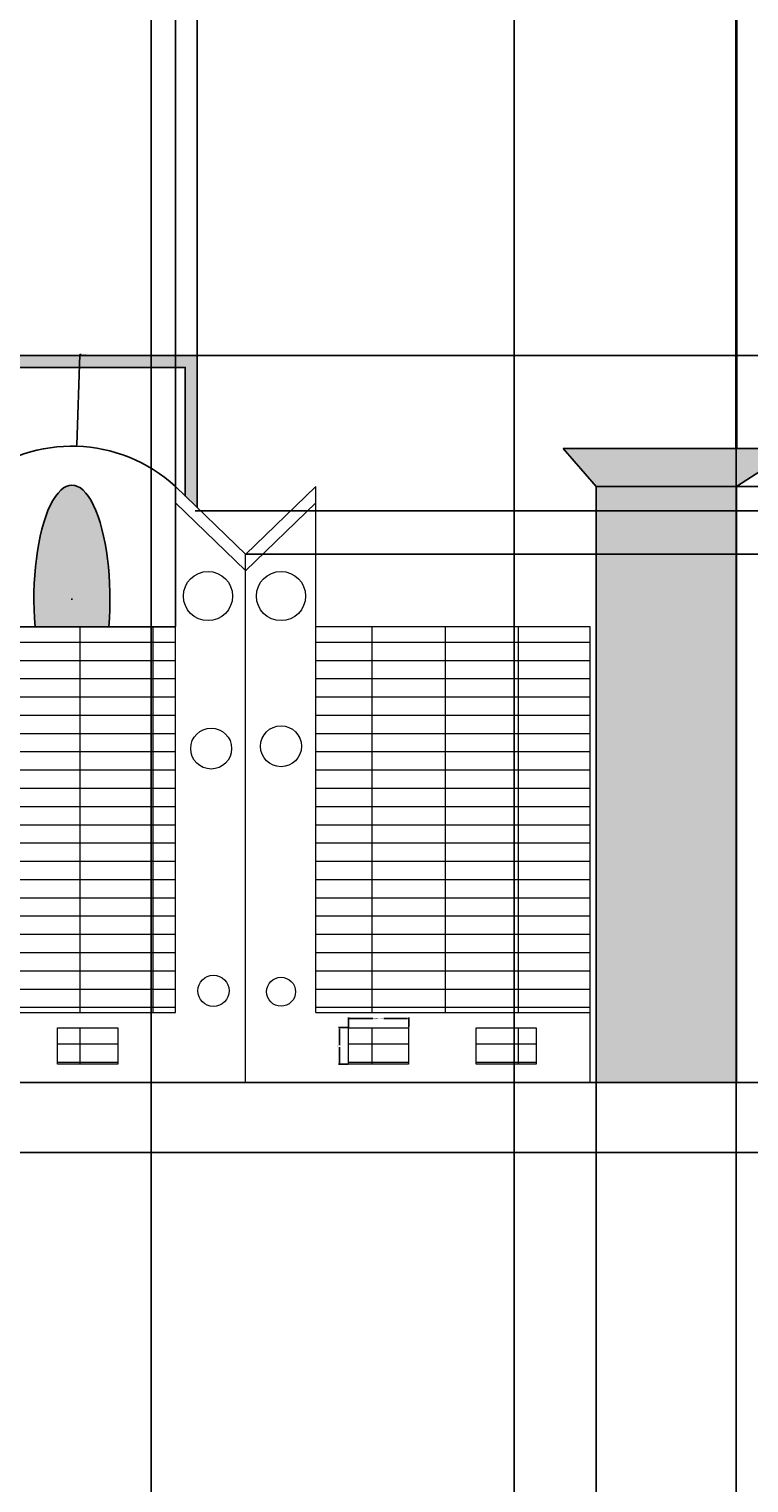
# Model space of a CAD drawing. Units: inches. Extents: x 484 to 1264, y 95 to 991.
# Tile 5 of 8: x 879 to 1002, y 250 to 499. Entities that reach past the tile are written whole.
import ezdxf

# ---------------------------------------------------------------- set-up
doc = ezdxf.new("R2010")
doc.units = ezdxf.units.IN
doc.header["$MEASUREMENT"] = 0
for name, color, linetype, lineweight in [('A-ANNO-DIMS', 2, 'Continuous', 18), ('A-DOOR', 7, 'Continuous', 25), ('A-WALL', 7, 'Continuous', 35), ('L-FENC', 7, 'Continuous', 25), ('L-FENC-GRIL-PATT', 6, 'Continuous', 13), ('L-GATE', 7, 'Continuous', 18)]:
    doc.layers.add(name, color=color, linetype=linetype, lineweight=lineweight)
doc.layers.add('A-ELEV-TRIM-PATT', color=40, linetype='Continuous', lineweight=13, true_color=0xe7c208)
doc.layers.add('L-FENC-PATT', color=34, linetype='Continuous', lineweight=13, true_color=0xa25420)
doc.styles.get("Standard").update_dxf_attribs({"font": 'arial.ttf'})
doc.dimstyles.get("Standard").update_dxf_attribs({"dimtxt": 0.18, "dimasz": 0.18, "dimexe": 0.18, "dimexo": 0.0625, "dimgap": 0.09, "dimtad": 0, "dimtih": 1, "dimtoh": 1, "dimdec": 4, "dimzin": 0, "dimdsep": 46, "dimtxsty": 'Standard', "dimcen": 0.09, "dimadec": 0, "dimazin": 0, "dimtfac": 1, "dimtdec": 4, "dimtofl": 0, "dimtmove": 0, "dimatfit": 3, "dimfxl": 1, "dimtolj": 1, "dimtzin": 0, "dimarcsym": 0})

# ---------------------------------------------------------------- blocks, each defined once
blk = doc.blocks.new('FENCE-PIER-CAP')
for p, q in [((5.63, 0), (0, 6.48)), ((0, 6.48), (39.71, 6.48)), ((39.71, 6.48), (29.63, 0))]:
    blk.add_line(p, q)
blk = doc.blocks.new('GATE-LOWER-INSET')
blk.add_lwpolyline([(0, 6.26), (10.31, 6.26), (10.31, 0), (0, 0)], close=True)
blk = doc.blocks.new('*D8')
at = {"layer": 'A-ANNO-DIMS', "color": 0, "lineweight": -2, "transparency": 16777216}
for p, q in [((933.42, 327.83), (933.42, 329.49)), ((933.6, 329.31), (937.65, 329.31)), ((943.55, 329.31), (939.5, 329.31)), ((943.73, 327.83), (943.73, 329.49))]:
    blk.add_line(p, q, dxfattribs=at)
at = {"layer": 'A-ANNO-DIMS', "color": 0, "transparency": 16777216}
for points in [[(933.6, 329.34), (933.6, 329.28), (933.42, 329.31)], [(943.55, 329.34), (943.55, 329.28), (943.73, 329.31)]]:
    blk.add_solid(points, dxfattribs=at)
at = {"layer": 'Defpoints', "color": 0, "transparency": 16777216}
for p in [(943.73, 329.31), (933.42, 327.77), (943.73, 327.77)]:
    blk.add_point(p, dxfattribs=at)
at = {"layer": 'A-ANNO-DIMS', "color": 0, "transparency": 16777216, "insert": (938.57, 329.31), "char_height": 0.18, "attachment_point": 5}
blk.add_mtext('\\A1;INSET 10 TYP.', dxfattribs=at)
blk = doc.blocks.new('*D9')
at = {"layer": 'A-ANNO-DIMS', "color": 0, "lineweight": -2, "transparency": 16777216}
for p, q in [((933.35, 327.77), (931.69, 327.77)), ((931.87, 327.59), (931.87, 324.82)), ((931.87, 321.68), (931.87, 324.45)), ((933.35, 321.5), (931.69, 321.5))]:
    blk.add_line(p, q, dxfattribs=at)
at = {"layer": 'A-ANNO-DIMS', "color": 0, "transparency": 16777216}
for points in [[(931.84, 327.59), (931.9, 327.59), (931.87, 327.77)], [(931.84, 321.68), (931.9, 321.68), (931.87, 321.5)]]:
    blk.add_solid(points, dxfattribs=at)
at = {"layer": 'Defpoints', "color": 0, "transparency": 16777216}
for p in [(931.87, 327.77), (933.42, 327.77), (933.42, 321.5)]:
    blk.add_point(p, dxfattribs=at)
at = {"layer": 'A-ANNO-DIMS', "color": 0, "transparency": 16777216, "insert": (931.87, 324.63), "char_height": 0.18, "attachment_point": 5}
blk.add_mtext('\\A1;6 TYP.', dxfattribs=at)
blk = doc.blocks.new('*D16')
at = {"layer": 'A-ANNO-DIMS', "color": 0, "lineweight": -2, "transparency": 16777216}
for p, q in [((639.81, 408.32), (639.81, 94.79)), ((999.81, 318.32), (999.81, 94.79)), ((639.99, 94.97), (819.53, 94.97)), ((999.63, 94.97), (820.1, 94.97))]:
    blk.add_line(p, q, dxfattribs=at)
at = {"layer": 'A-ANNO-DIMS', "color": 0, "transparency": 16777216}
for points in [[(639.99, 95), (639.99, 94.94), (639.81, 94.97)], [(999.63, 95), (999.63, 94.94), (999.81, 94.97)]]:
    blk.add_solid(points, dxfattribs=at)
at = {"layer": 'Defpoints', "color": 0, "transparency": 16777216}
for p in [(639.81, 408.38), (999.81, 318.38), (999.81, 94.97)]:
    blk.add_point(p, dxfattribs=at)
at = {"layer": 'A-ANNO-DIMS', "color": 0, "transparency": 16777216, "insert": (819.81, 94.97), "char_height": 0.18, "attachment_point": 5}
blk.add_mtext('\\A1;360', dxfattribs=at)
blk = doc.blocks.new('*D18')
at = {"layer": 'A-ANNO-DIMS', "color": 0, "lineweight": -2, "transparency": 16777216}
for p, q in [((999.88, 501.38), (1264.08, 501.38)), ((1263.9, 501.2), (1263.9, 404.07)), ((1263.9, 306.56), (1263.9, 403.7)), ((595.38, 306.38), (1264.08, 306.38))]:
    blk.add_line(p, q, dxfattribs=at)
at = {"layer": 'A-ANNO-DIMS', "color": 0, "transparency": 16777216}
for points in [[(1263.87, 501.2), (1263.93, 501.2), (1263.9, 501.38)], [(1263.87, 306.56), (1263.93, 306.56), (1263.9, 306.38)]]:
    blk.add_solid(points, dxfattribs=at)
at = {"layer": 'Defpoints', "color": 0, "transparency": 16777216}
for p in [(999.81, 501.38), (1263.9, 501.38), (595.32, 306.38)]:
    blk.add_point(p, dxfattribs=at)
at = {"layer": 'A-ANNO-DIMS', "color": 0, "transparency": 16777216, "insert": (1263.9, 403.88), "char_height": 0.18, "attachment_point": 5}
blk.add_mtext('\\A1;195', dxfattribs=at)
blk = doc.blocks.new('*D40')
at = {"layer": 'A-ANNO-DIMS', "color": 0, "lineweight": -2, "transparency": 16777216}
for p, q in [((899.68, 562.19), (899.68, 94.79)), ((961.76, 562.19), (961.76, 94.79)), ((899.86, 94.97), (930.33, 94.97)), ((961.58, 94.97), (931.12, 94.97))]:
    blk.add_line(p, q, dxfattribs=at)
at = {"layer": 'A-ANNO-DIMS', "color": 0, "transparency": 16777216}
for points in [[(899.86, 95), (899.86, 94.94), (899.68, 94.97)], [(961.58, 95), (961.58, 94.94), (961.76, 94.97)]]:
    blk.add_solid(points, dxfattribs=at)
at = {"layer": 'Defpoints', "color": 0, "transparency": 16777216}
for p in [(899.68, 562.26), (961.76, 562.26), (961.76, 94.97)]:
    blk.add_point(p, dxfattribs=at)
at = {"layer": 'A-ANNO-DIMS', "color": 0, "transparency": 16777216, "insert": (930.72, 94.97), "char_height": 0.18, "attachment_point": 5}
blk.add_mtext('\\A1;62.08', dxfattribs=at)
blk = doc.blocks.new('*D41')
at = {"layer": 'A-ANNO-DIMS', "color": 0, "lineweight": -2, "transparency": 16777216}
for p, q in [((961.76, 562.19), (961.76, 94.79)), ((999.81, 537.32), (999.81, 94.79)), ((961.94, 94.97), (980.39, 94.97)), ((999.63, 94.97), (981.18, 94.97))]:
    blk.add_line(p, q, dxfattribs=at)
at = {"layer": 'A-ANNO-DIMS', "color": 0, "transparency": 16777216}
for points in [[(961.94, 95), (961.94, 94.94), (961.76, 94.97)], [(999.63, 95), (999.63, 94.94), (999.81, 94.97)]]:
    blk.add_solid(points, dxfattribs=at)
at = {"layer": 'Defpoints', "color": 0, "transparency": 16777216}
for p in [(961.76, 562.26), (999.81, 537.38), (999.81, 94.97)]:
    blk.add_point(p, dxfattribs=at)
at = {"layer": 'A-ANNO-DIMS', "color": 0, "transparency": 16777216, "insert": (980.79, 94.97), "char_height": 0.18, "attachment_point": 5}
blk.add_mtext('\\A1;38.05', dxfattribs=at)
blk = doc.blocks.new('*D49')
at = {"layer": 'A-ANNO-DIMS', "color": 0, "lineweight": -2, "transparency": 16777216}
for p, q in [((855.81, 318.32), (855.81, 94.79)), ((975.81, 318.32), (975.81, 94.79)), ((855.99, 94.97), (915.53, 94.97)), ((975.63, 94.97), (916.09, 94.97))]:
    blk.add_line(p, q, dxfattribs=at)
at = {"layer": 'A-ANNO-DIMS', "color": 0, "transparency": 16777216}
for points in [[(855.99, 95), (855.99, 94.94), (855.81, 94.97)], [(975.63, 95), (975.63, 94.94), (975.81, 94.97)]]:
    blk.add_solid(points, dxfattribs=at)
at = {"layer": 'Defpoints', "color": 0, "transparency": 16777216}
for p in [(855.81, 318.38), (975.81, 318.38), (975.81, 94.97)]:
    blk.add_point(p, dxfattribs=at)
at = {"layer": 'A-ANNO-DIMS', "color": 0, "transparency": 16777216, "insert": (915.81, 94.97), "char_height": 0.18, "attachment_point": 5}
blk.add_mtext('\\A1;120', dxfattribs=at)
blk = doc.blocks.new('*D50')
at = {"layer": 'A-ANNO-DIMS', "color": 0, "lineweight": -2, "transparency": 16777216}
for p, q in [((999.88, 420.38), (1264.08, 420.38)), ((1263.9, 420.2), (1263.9, 369.57)), ((1263.9, 318.56), (1263.9, 369.2)), ((999.88, 318.38), (1264.08, 318.38))]:
    blk.add_line(p, q, dxfattribs=at)
at = {"layer": 'A-ANNO-DIMS', "color": 0, "transparency": 16777216}
for points in [[(1263.87, 420.2), (1263.93, 420.2), (1263.9, 420.38)], [(1263.87, 318.56), (1263.93, 318.56), (1263.9, 318.38)]]:
    blk.add_solid(points, dxfattribs=at)
at = {"layer": 'Defpoints', "color": 0, "transparency": 16777216}
for p in [(999.81, 420.38), (1263.9, 420.38), (999.81, 318.38)]:
    blk.add_point(p, dxfattribs=at)
at = {"layer": 'A-ANNO-DIMS', "color": 0, "transparency": 16777216, "insert": (1263.9, 369.38), "char_height": 0.18, "attachment_point": 5}
blk.add_mtext('\\A1;102', dxfattribs=at)
blk = doc.blocks.new('*D55')
at = {"layer": 'A-ANNO-DIMS', "color": 0, "lineweight": -2, "transparency": 16777216}
for p, q in [((975.81, 318.32), (975.81, 94.79)), ((999.81, 318.32), (999.81, 94.79)), ((975.99, 94.97), (987.59, 94.97)), ((999.63, 94.97), (988.03, 94.97))]:
    blk.add_line(p, q, dxfattribs=at)
at = {"layer": 'A-ANNO-DIMS', "color": 0, "transparency": 16777216}
for points in [[(975.99, 95), (975.99, 94.94), (975.81, 94.97)], [(999.63, 95), (999.63, 94.94), (999.81, 94.97)]]:
    blk.add_solid(points, dxfattribs=at)
at = {"layer": 'Defpoints', "color": 0, "transparency": 16777216}
for p in [(975.81, 318.38), (999.81, 318.38), (999.81, 94.97)]:
    blk.add_point(p, dxfattribs=at)
at = {"layer": 'A-ANNO-DIMS', "color": 0, "transparency": 16777216, "insert": (987.81, 94.97), "char_height": 0.18, "attachment_point": 5}
blk.add_mtext('\\A1;24', dxfattribs=at)
blk = doc.blocks.new('*D56')
at = {"layer": 'A-ANNO-DIMS', "color": 0, "lineweight": -2, "transparency": 16777216}
for p, q in [((915.88, 408.78), (1264.08, 408.78)), ((1263.9, 408.6), (1263.9, 363.76)), ((1263.9, 318.56), (1263.9, 363.4)), ((915.88, 318.38), (1264.08, 318.38))]:
    blk.add_line(p, q, dxfattribs=at)
at = {"layer": 'A-ANNO-DIMS', "color": 0, "transparency": 16777216}
for points in [[(1263.87, 408.6), (1263.93, 408.6), (1263.9, 408.78)], [(1263.87, 318.56), (1263.93, 318.56), (1263.9, 318.38)]]:
    blk.add_solid(points, dxfattribs=at)
at = {"layer": 'Defpoints', "color": 0, "transparency": 16777216}
for p in [(915.81, 408.78), (1263.9, 408.78), (915.81, 318.38)]:
    blk.add_point(p, dxfattribs=at)
at = {"layer": 'A-ANNO-DIMS', "color": 0, "transparency": 16777216, "insert": (1263.9, 363.58), "char_height": 0.18, "attachment_point": 5}
blk.add_mtext('\\A1;90.4', dxfattribs=at)
blk = doc.blocks.new('*D57')
at = {"layer": 'A-ANNO-DIMS', "color": 0, "lineweight": -2, "transparency": 16777216}
for p, q in [((855.81, 396.45), (855.81, 991.11)), ((855.99, 990.93), (879.59, 990.93)), ((903.63, 990.93), (880.04, 990.93)), ((903.81, 396.45), (903.81, 991.11))]:
    blk.add_line(p, q, dxfattribs=at)
at = {"layer": 'A-ANNO-DIMS', "color": 0, "transparency": 16777216}
for points in [[(855.99, 990.96), (855.99, 990.9), (855.81, 990.93)], [(903.63, 990.96), (903.63, 990.9), (903.81, 990.93)]]:
    blk.add_solid(points, dxfattribs=at)
at = {"layer": 'Defpoints', "color": 0, "transparency": 16777216}
for p in [(903.81, 990.93), (855.81, 396.38), (903.81, 396.38)]:
    blk.add_point(p, dxfattribs=at)
at = {"layer": 'A-ANNO-DIMS', "color": 0, "transparency": 16777216, "insert": (879.81, 990.93), "char_height": 0.18, "attachment_point": 5}
blk.add_mtext('\\A1;48', dxfattribs=at)
blk = doc.blocks.new('*D59')
at = {"layer": 'A-ANNO-DIMS', "color": 0, "lineweight": -2, "transparency": 16777216}
for p, q in [((855.88, 318.38), (1264.08, 318.38)), ((1263.9, 318.2), (1263.9, 312.56)), ((1263.9, 306.56), (1263.9, 312.2)), ((855.88, 306.38), (1264.08, 306.38))]:
    blk.add_line(p, q, dxfattribs=at)
at = {"layer": 'A-ANNO-DIMS', "color": 0, "transparency": 16777216}
for points in [[(1263.87, 318.2), (1263.93, 318.2), (1263.9, 318.38)], [(1263.87, 306.56), (1263.93, 306.56), (1263.9, 306.38)]]:
    blk.add_solid(points, dxfattribs=at)
at = {"layer": 'Defpoints', "color": 0, "transparency": 16777216}
for p in [(855.81, 318.38), (855.81, 306.38), (1263.9, 306.38)]:
    blk.add_point(p, dxfattribs=at)
at = {"layer": 'A-ANNO-DIMS', "color": 0, "transparency": 16777216, "insert": (1263.9, 312.38), "char_height": 0.18, "attachment_point": 5}
blk.add_mtext('\\A1;12', dxfattribs=at)
blk = doc.blocks.new('*D61')
at = {"layer": 'A-ANNO-DIMS', "color": 0, "lineweight": -2, "transparency": 16777216}
for p, q in [((855.81, 396.45), (855.81, 991.11)), ((855.99, 990.93), (881.26, 990.93)), ((907.32, 990.93), (882.05, 990.93)), ((907.5, 442.84), (907.5, 991.11))]:
    blk.add_line(p, q, dxfattribs=at)
at = {"layer": 'A-ANNO-DIMS', "color": 0, "transparency": 16777216}
for points in [[(855.99, 990.96), (855.99, 990.9), (855.81, 990.93)], [(907.32, 990.96), (907.32, 990.9), (907.5, 990.93)]]:
    blk.add_solid(points, dxfattribs=at)
at = {"layer": 'Defpoints', "color": 0, "transparency": 16777216}
for p in [(907.5, 990.93), (907.5, 442.78), (855.81, 396.38)]:
    blk.add_point(p, dxfattribs=at)
at = {"layer": 'A-ANNO-DIMS', "color": 0, "transparency": 16777216, "insert": (881.66, 990.93), "char_height": 0.18, "attachment_point": 5}
blk.add_mtext('\\A1;51.68', dxfattribs=at)
blk = doc.blocks.new('*D62')
at = {"layer": 'A-ANNO-DIMS', "color": 0, "lineweight": -2, "transparency": 16777216}
for p, q in [((907.56, 442.78), (1264.08, 442.78)), ((1263.9, 442.6), (1263.9, 429.68)), ((1263.9, 416.4), (1263.9, 429.32)), ((907.18, 416.22), (1264.08, 416.22))]:
    blk.add_line(p, q, dxfattribs=at)
at = {"layer": 'A-ANNO-DIMS', "color": 0, "transparency": 16777216}
for points in [[(1263.87, 442.6), (1263.93, 442.6), (1263.9, 442.78)], [(1263.87, 416.4), (1263.93, 416.4), (1263.9, 416.22)]]:
    blk.add_solid(points, dxfattribs=at)
at = {"layer": 'Defpoints', "color": 0, "transparency": 16777216}
for p in [(907.5, 442.78), (907.12, 416.22), (1263.9, 416.22)]:
    blk.add_point(p, dxfattribs=at)
at = {"layer": 'A-ANNO-DIMS', "color": 0, "transparency": 16777216, "insert": (1263.9, 429.5), "char_height": 0.18, "attachment_point": 5}
blk.add_mtext('\\A1;26.56', dxfattribs=at)
blk = doc.blocks.new('*D63')
at = {"layer": 'A-ANNO-DIMS', "color": 0, "lineweight": -2, "transparency": 16777216}
for p, q in [((887.42, 443), (886.92, 427.46)), ((887.6, 443), (887.42, 443)), ((885.99, 401.09), (886.17, 401.09)), ((886.08, 401), (886.08, 401.18))]:
    blk.add_line(p, q, dxfattribs=at)
at = {"layer": 'A-ANNO-DIMS', "color": 0, "transparency": 16777216}
blk.add_solid([(886.89, 427.46), (886.95, 427.46), (886.92, 427.28)], dxfattribs=at)
at = {"layer": 'Defpoints', "color": 0, "transparency": 16777216}
for p in [(886.92, 427.28), (886.08, 401.09)]:
    blk.add_point(p, dxfattribs=at)
at = {"layer": 'A-ANNO-DIMS', "color": 0, "transparency": 16777216, "insert": (888.15, 443), "char_height": 0.18, "attachment_point": 5}
blk.add_mtext('\\A1;R26.203', dxfattribs=at)

msp = doc.modelspace()

# ---------------------------------------------------------------- hatches: boundary and pattern name
at = {"layer": 'A-ELEV-TRIM-PATT'}
h = msp.add_hatch(color=256, dxfattribs=at)
h.dxf.hatch_style = 1
h.paths.add_polyline_path([(629.3986, 426.86), (589.6936, 426.86), (595.3221, 420.3846), (619.3221, 420.3846)])
edge = h.paths.add_edge_path()
edge.add_line((857.8147, 421.9731), (857.8147, 421.9373))
edge.add_ellipse((838.7195, 429.7418), major_axis=(-35.8241, 0), ratio=0.25748145, start_angle=157.76958, end_angle=158.416192)
edge.add_line((858.2614, 422.011), (865.8912, 426.9141))
edge.add_line((865.8912, 426.9141), (826.1862, 426.9141))
edge.add_line((826.1862, 426.9141), (831.8617, 420.3846))
edge.add_line((831.8617, 420.3846), (855.7305, 420.3846))
edge.add_line((855.7305, 420.3846), (856.3445, 420.7792))
edge.add_line((856.3445, 420.7792), (857.8147, 421.9731))
h.paths.add_polyline_path([(1009.8912, 426.86), (970.1862, 426.86), (975.8147, 420.3846), (999.8147, 420.3846)])
h.paths.add_polyline_path([(857.8147, 421.7239), (856.3445, 420.7792), (855.8147, 420.3489), (855.8147, 396.3846), (857.8147, 396.3846)])
edge = h.paths.add_edge_path()
edge.add_ellipse((838.7195, 448.4615), major_axis=(-35.8241, 0), ratio=0.25748145, start_angle=154.631086, end_angle=157.76958, ccw=False)
edge.add_line((855.8147, 440.3555), (855.8147, 437.8478))
edge.add_ellipse((838.7195, 429.7418), major_axis=(-35.8241, 0), ratio=0.25748145, start_angle=202.23042, end_angle=205.368914, ccw=False)
edge.add_line((857.8147, 437.5462), (857.8147, 440.6571))
edge = h.paths.add_edge_path()
edge.add_line((907.4984, 442.7783), (866.9359, 442.7783))
edge.add_ellipse((838.7195, 448.4615), major_axis=(-35.8241, 0), ratio=0.25748145, start_angle=158.813461, end_angle=168.611984, ccw=False)
edge.add_line((858.542, 440.7783), (905.4984, 440.7783))
edge.add_line((905.4984, 440.7783), (905.4984, 418.7562))
edge.add_line((905.4984, 418.7562), (907.4984, 416.8218))
edge.add_line((907.4984, 416.8218), (907.4984, 442.7783))
h = msp.add_hatch(color=256, dxfattribs=at)
h.dxf.hatch_style = 1
edge = h.paths.add_edge_path()
edge.add_ellipse((886.0837, 401.0921), major_axis=(0, 19.5309), ratio=0.33293274, start_angle=233.278842, end_angle=486.721158)
edge.add_line((879.773, 396.3846), (892.3945, 396.3846))
at = {"layer": 'L-FENC-GRIL-PATT'}
h = msp.add_hatch(dxfattribs=at)
h.set_pattern_fill('GRATE', color=256, scale=100)
h.paths.add_polyline_path([(974.8147, 396.3846), (927.8147, 396.3846), (927.8147, 330.3846), (974.8147, 330.3846)])
h.paths.add_polyline_path([(903.8147, 396.3846), (855.8147, 396.3846), (855.8147, 330.3846), (903.8147, 330.3846)])
h.paths.add_polyline_path([(819.8147, 420.3846), (807.8147, 420.3846), (807.8147, 408.3846), (819.8147, 408.3846)])
h.paths.add_polyline_path([(807.8147, 420.3846), (795.8147, 420.3846), (795.8147, 408.3846), (807.8147, 408.3846)])
h.paths.add_polyline_path([(795.8147, 420.3846), (783.8147, 420.3846), (783.8147, 408.3846), (795.8147, 408.3846)])
h.paths.add_polyline_path([(831.8147, 420.3846), (819.8147, 420.3846), (819.8147, 408.3846), (831.8147, 408.3846)])
h.paths.add_polyline_path([(783.8147, 420.3846), (779.9105, 420.3846), (779.9105, 412.138), (771.8147, 412.138), (771.8147, 408.3846), (783.8147, 408.3846)])
h.paths.add_polyline_path([(777.9105, 420.3846), (771.8147, 420.3846), (771.8147, 414.138), (777.9105, 414.138)], flags=17)
h.paths.add_polyline_path([(723.8147, 420.3846), (711.8147, 420.3846), (711.8147, 408.3846), (723.8147, 408.3846)])
h.paths.add_polyline_path([(711.8147, 420.3846), (699.8147, 420.3846), (699.8147, 408.3846), (711.8147, 408.3846)])
h.paths.add_polyline_path([(699.8147, 420.3846), (687.8147, 420.3846), (687.8147, 408.3846), (699.8147, 408.3846)])
h.paths.add_polyline_path([(687.8147, 420.3846), (675.8147, 420.3846), (675.8147, 408.3846), (687.8147, 408.3846)])
h.paths.add_polyline_path([(675.8147, 420.3846), (663.8147, 420.3846), (663.8147, 408.3846), (675.8147, 408.3846)])
h.paths.add_polyline_path([(639.8147, 420.3846), (631.3221, 420.3846), (631.3221, 408.3846), (639.8147, 408.3846)])
h.paths.add_polyline_path([(631.3221, 420.3846), (619.3221, 420.3846), (619.3221, 408.3846), (631.3221, 408.3846)])
h = msp.add_hatch(dxfattribs=at)
h.set_pattern_fill('GRATE', color=256, scale=100)
h.paths.add_polyline_path([(965.5846, 327.7657), (955.27, 327.7657), (955.27, 321.5012), (965.5846, 321.5012)])
h.paths.add_polyline_path([(943.7309, 327.7657), (933.4163, 327.7657), (933.4163, 321.5012), (943.7309, 321.5012)])
h.paths.add_polyline_path([(893.9522, 327.7657), (883.6376, 327.7657), (883.6376, 321.5012), (893.9522, 321.5012)])
h.paths.add_polyline_path([(872.1278, 327.7657), (861.8132, 327.7657), (861.8132, 321.5012), (872.1278, 321.5012)])
at = {"layer": 'L-FENC-PATT'}
h = msp.add_hatch(color=256, dxfattribs=at)
h.dxf.hatch_style = 1
h.paths.add_polyline_path([(619.3221, 420.3846), (595.3221, 420.3846), (595.3221, 306.3846), (855.8147, 306.3846), (855.8147, 420.3846), (831.8147, 420.3846), (831.8147, 330.3846), (771.8147, 330.3846), (771.8147, 420.3846), (723.8147, 420.3846), (723.8147, 330.3846), (619.3221, 330.3846)])
h.paths.add_polyline_path([(999.8147, 420.3846), (975.8147, 420.3846), (975.8147, 318.3846), (999.8147, 318.3846)])

# ---------------------------------------------------------------- linework, layer by layer
at = {"layer": 'A-DOOR'}
for points in [[(905.4984, 418.7562), (905.4984, 440.7783), (858.542, 440.7783)], [(907.4984, 416.8218), (907.4984, 442.7783), (866.9359, 442.7783)], [(855.8147, 420.3846), (855.8147, 396.3846), (903.8147, 396.3846)]]:
    msp.add_lwpolyline(points, dxfattribs=at)
msp.add_arc((886.0837, 401.0921), 26.2028, 47.415078, 128.940912, dxfattribs=at)
msp.add_ellipse((886.0837, 401.0921), major_axis=(0, 19.5309), ratio=0.33293274, start_param=4.46896224, end_param=8.09740837, dxfattribs=at)
at = {"layer": 'A-WALL'}
msp.add_line((999.8147, 426.86), (999.8147, 810.3846), dxfattribs=at)
at = {"layer": 'L-FENC'}
for p, q in [((999.8147, 420.3846), (975.8147, 420.3846)), ((975.8147, 318.3846), (975.8147, 420.3846)), ((999.8147, 318.3846), (999.8147, 420.3846))]:
    msp.add_line(p, q, dxfattribs=at)
at = {"layer": 'L-GATE'}
for p, q in [((903.8147, 330.3846), (903.8147, 420.3846)), ((903.8147, 420.3846), (915.8368, 408.7571)), ((927.8147, 420.3846), (915.8147, 408.7356)), ((927.8147, 330.3846), (927.8147, 420.3846)), ((903.8147, 417.6022), (915.8147, 405.9961)), ((927.8147, 417.5972), (915.8147, 405.9482)), ((915.8147, 318.3846), (915.8147, 408.7785)), ((903.8147, 396.3846), (855.8147, 396.3846)), ((974.8147, 396.3846), (927.8147, 396.3846)), ((974.8147, 318.3846), (974.8147, 396.3846)), ((855.8147, 330.3846), (903.8147, 330.3846)), ((927.8147, 330.3846), (974.8147, 330.3846)), ((855.8147, 318.3846), (999.8147, 318.3846))]:
    msp.add_line(p, q, dxfattribs=at)
for centre, radius in [((909.3805, 401.6332), 4.2058), ((921.8762, 401.6332), 4.2058), ((909.924, 375.5281), 3.5014), ((921.8762, 375.924), 3.5014), ((910.306, 334.076), 2.6771), ((921.8762, 333.9174), 2.4781)]:
    msp.add_circle(centre, radius, dxfattribs=at)

# ---------------------------------------------------------------- block references
at = {"layer": 'L-FENC'}
msp.add_blockref('FENCE-PIER-CAP', (970.1862, 420.3846), dxfattribs=at)
at = {"layer": 'L-GATE'}
for p in [(883.6376, 321.5012), (933.4163, 321.5012), (955.27, 321.5012)]:
    msp.add_blockref('GATE-LOWER-INSET', p, dxfattribs=at)

# ---------------------------------------------------------------- dimensions: what is measured, and where the dimension line sits
at = {"layer": 'A-ANNO-DIMS'}
for base, p1, p2, override, picture, middle in [((903.8147, 990.929), (855.8147, 396.3846), (903.8147, 396.3846), {"dimdec": 0, "dimlfac": 1, "dimrnd": 0, "dimzin": 0, "dimdsep": 46, "dimlunit": 2}, '*D57', (879.8147, 990.929)), ((907.4984, 990.929), (855.8147, 396.3846), (907.4984, 442.7783), {"dimdec": 2, "dimlfac": 1, "dimrnd": 0, "dimzin": 0, "dimdsep": 46, "dimlunit": 2}, '*D61', (881.6566, 990.929)), ((961.7639, 94.9714), (899.6817, 562.256), (961.7639, 562.256), {"dimdec": 2, "dimlfac": 1, "dimrnd": 0, "dimzin": 0, "dimdsep": 46, "dimlunit": 2}, '*D40', (930.7228, 94.9714)), ((999.8147, 94.9714), (961.7639, 562.256), (999.8147, 537.3846), {"dimdec": 2, "dimlfac": 1, "dimrnd": 0, "dimzin": 0, "dimdsep": 46, "dimlunit": 2}, '*D41', (980.7893, 94.9714)), ((999.8147, 94.9714), (639.8147, 408.3846), (999.8147, 318.3846), {"dimdec": 0, "dimlfac": 1, "dimrnd": 0, "dimzin": 0, "dimdsep": 46, "dimlunit": 2}, '*D16', (819.8147, 94.9714)), ((975.8147, 94.9714), (855.8147, 318.3846), (975.8147, 318.3846), {"dimdec": 0, "dimlfac": 1, "dimrnd": 0, "dimzin": 0, "dimdsep": 46, "dimlunit": 2}, '*D49', (915.8147, 94.9714)), ((999.8147, 94.9714), (975.8147, 318.3846), (999.8147, 318.3846), {"dimdec": 0, "dimlfac": 1, "dimrnd": 0, "dimzin": 0, "dimdsep": 46, "dimlunit": 2}, '*D55', (987.8147, 94.9714))]:
    dim = msp.add_linear_dim(base=base, p1=p1, p2=p2, dimstyle='Standard', override=override, dxfattribs=at)
    dim.commit()
    dim.dimension.update_dxf_attribs({"geometry": picture, "text_midpoint": middle})
for base, p1, p2, override, picture, middle in [((1263.9032, 501.3846), (595.3221, 306.3846), (999.8147, 501.3846), {"dimdec": 0, "dimlfac": 1, "dimrnd": 0, "dimzin": 0, "dimdsep": 46, "dimlunit": 2}, '*D18', (1263.9032, 403.8846)), ((1263.9032, 416.2209), (907.4984, 442.7783), (907.1219, 416.2209), {"dimdec": 2, "dimlfac": 1, "dimrnd": 0, "dimzin": 0, "dimdsep": 46, "dimlunit": 2}, '*D62', (1263.9032, 429.4996)), ((1263.9032, 420.3846), (999.8147, 318.3846), (999.8147, 420.3846), {"dimdec": 0, "dimlfac": 1, "dimrnd": 0, "dimzin": 0, "dimdsep": 46, "dimlunit": 2}, '*D50', (1263.9032, 369.3846)), ((1263.9032, 408.7785), (915.8147, 318.3846), (915.8147, 408.7785), {"dimdec": 1, "dimlfac": 1, "dimrnd": 0, "dimzin": 0, "dimdsep": 46, "dimlunit": 2}, '*D56', (1263.9032, 363.5815)), ((1263.9032, 306.3846), (855.8147, 318.3846), (855.8147, 306.3846), {"dimdec": 0, "dimlfac": 1, "dimrnd": 0, "dimzin": 0, "dimdsep": 46, "dimlunit": 2}, '*D59', (1263.9032, 312.3846))]:
    dim = msp.add_linear_dim(base=base, p1=p1, p2=p2, angle=90, dimstyle='Standard', override=override, dxfattribs=at)
    dim.commit()
    dim.dimension.update_dxf_attribs({"geometry": picture, "text_midpoint": middle})
dim = msp.add_radius_dim(center=(886.0837, 401.0921), mpoint=(886.917, 427.2817), dimstyle='Standard', override={"dimdec": 3, "dimlfac": 1, "dimrnd": 0, "dimzin": 0, "dimdsep": 46, "dimlunit": 2}, dxfattribs=at)
dim.commit()
dim.dimension.update_dxf_attribs({"geometry": '*D63', "text_midpoint": (888.1467, 442.9954), "dimtype": 164})
dim = msp.add_linear_dim(base=(943.7309, 329.3129), p1=(933.4163, 327.7657), p2=(943.7309, 327.7657), text='INSET <> TYP.', dimstyle='Standard', override={"dimdec": 0, "dimlfac": 1, "dimrnd": 0, "dimzin": 0, "dimdsep": 46, "dimlunit": 2}, dxfattribs=at)
dim.commit()
dim.dimension.update_dxf_attribs({"geometry": '*D8', "text_midpoint": (938.5736, 329.3129)})
dim = msp.add_linear_dim(base=(931.8691, 327.7657), p1=(933.4163, 321.5012), p2=(933.4163, 327.7657), angle=90, text='<> TYP.', dimstyle='Standard', override={"dimdec": 0, "dimlfac": 1, "dimrnd": 0, "dimzin": 0, "dimdsep": 46, "dimlunit": 2}, dxfattribs=at)
dim.commit()
dim.dimension.update_dxf_attribs({"geometry": '*D9', "text_midpoint": (931.8691, 324.6334)})

doc.saveas('drawing.dxf')
